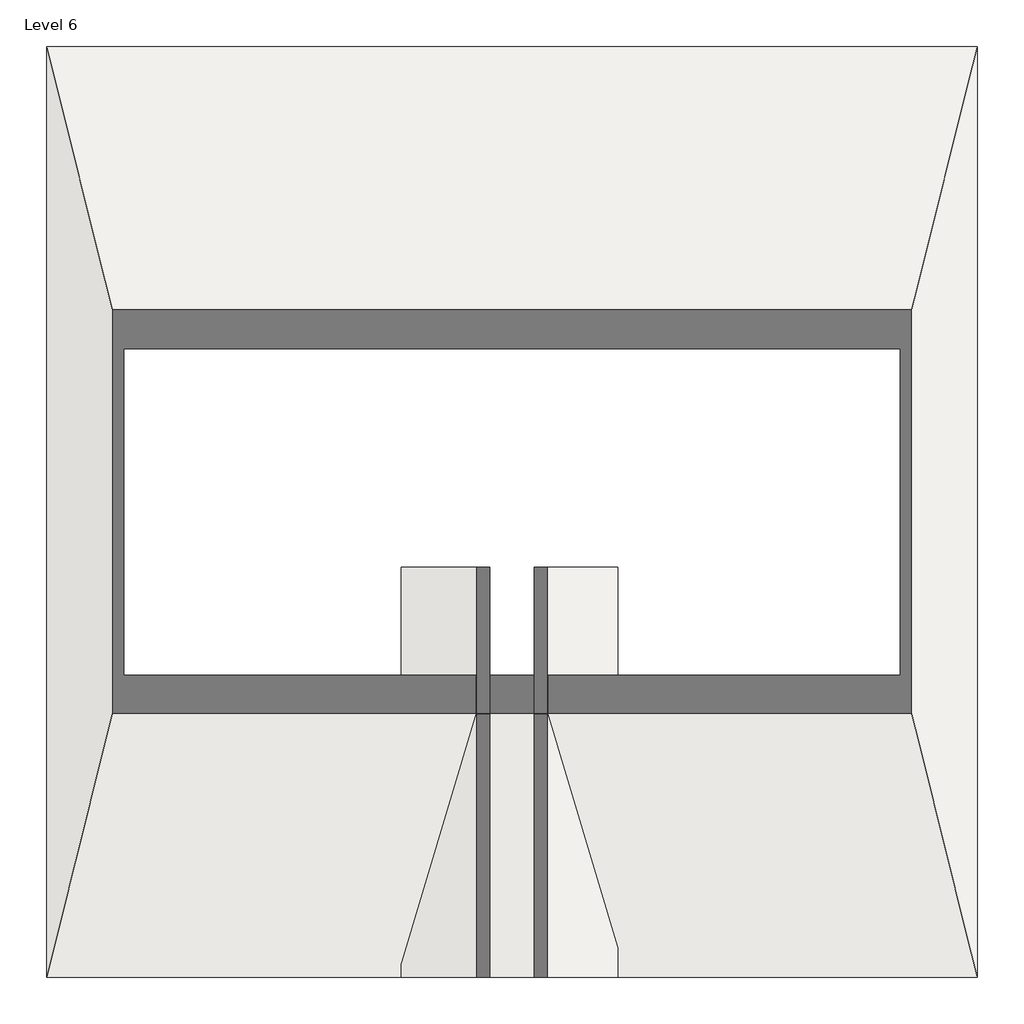
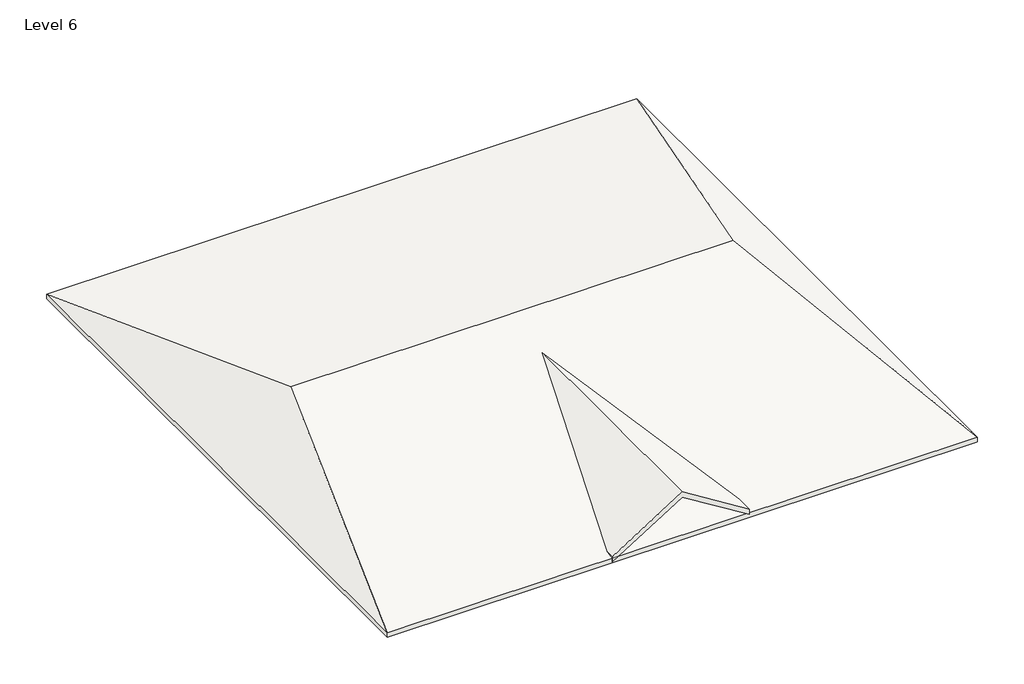
# One storey: 2 roofs.
"""IFC4 building model written with IfcOpenShell, lengths in millimetres."""

from ifc_helpers import new_model, si_unit, frame, origin, place, context, project, spatial, polyline, outline, extrude, faceted_brep, element, save

model = new_model("IFC4")

# Units and contexts
model_context = context("Model", 3, world=origin())
ifc_project = project(units=[si_unit("LENGTHUNIT", "METRE", prefix="MILLI")], contexts=[model_context])

# Site, building, storey
site = spatial("IfcSite", under=ifc_project)
building = spatial("IfcBuilding", under=site)
storey = spatial("IfcBuildingStorey", under=building, Name="Level 6", Elevation=7061.2)

# Roofs
placement = place(None, origin())
element("IfcRoof", 1, ObjectType="6\" roof", at=placement, inside=storey, context=model_context, shape_type="Brep", body=[
    faceted_brep([(9308.4836181, 9587.3121658, 7061.2), (6846.9031808, -280.5878342, 8907.385328), (-7871.1873126, -280.5878342, 8907.385328), (-10332.7677499, 9587.3121658, 7061.2), (-10332.7677499, -10148.4878342, 7061.2), (9308.4836181, -10148.4878342, 7061.2), (9355.7579341, 9587.3121658, 7216.244263), (-10380.0420659, 9587.3121658, 7216.244263), (-7918.4616286, -280.5878342, 9062.429591), (6894.1774968, -280.5878342, 9062.429591), (-10380.0420659, -10148.4878342, 7216.244263), (9355.7579341, -10148.4878342, 7216.244263), (-10380.0420659, 9587.3121658, 7061.2), (9355.7579341, 9587.3121658, 7061.2), (-10380.0420659, -10148.4878342, 7061.2), (9355.7579341, -10148.4878342, 7061.2)], [[[0, 1, 2, 3]], [[3, 2, 4]], [[4, 2, 1, 5]], [[1, 0, 5]], [[6, 7, 8, 9]], [[7, 10, 8]], [[10, 11, 9, 8]], [[6, 9, 11]], [[12, 7, 6, 13, 0, 3]], [[14, 10, 7, 12]], [[15, 11, 10, 14, 4, 5]], [[13, 6, 11, 15]], [[13, 15, 5, 0]], [[4, 14, 12, 3]]]),
])
element("IfcRoof", 2, ObjectType="6\" roof", at=placement, inside=storey, context=model_context, shape_type="SweptSolid", body=[
    extrude(outline(polyline([(7270.465525, -2860.0480249), (7090.7587364, -2860.0480249), (8557.8932113, -512.1420659), (7158.0584829, 1728.0617849), (7337.7652716, 1728.0617849), (8737.6, -512.1420659), (7270.465525, -2860.0480249)])), frame((0.0, -10148.4878342, 0.0), z_axis=(0.0, 1.0, 0.0), x_axis=(0.0, 0.0, 1.0)), (0.0, 0.0, 1.0), 8696.0664764),
])

save(model, "model.ifc")

# Revit data of these elements
# Type "6\" roof"
#   Assembly Code = "B1020"
#   Layers, outside or top first: 0' - 6" "roof balcony" (function 1)
# Element 1 (IfcRoof, "6\" roof")
#   built-in parameter 1001705 = 29.7324 (stored number, unit not read)
#   built-in parameter 1001710 = 33615
#   Phase Created = New Construction
#   Materials on its faces: "roof balcony"
# Element 2 (IfcRoof, "6\" roof")
#   built-in parameter 1001710 = 33615
#   Phase Created = New Construction
#   Materials on its faces: "roof balcony"
# Materials
#   "roof balcony": class "Generic", colour RGB 120 120 120, transparency 0, Cost = 0
